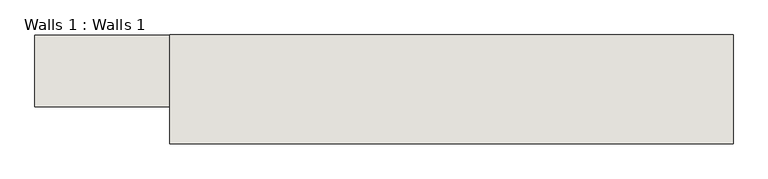
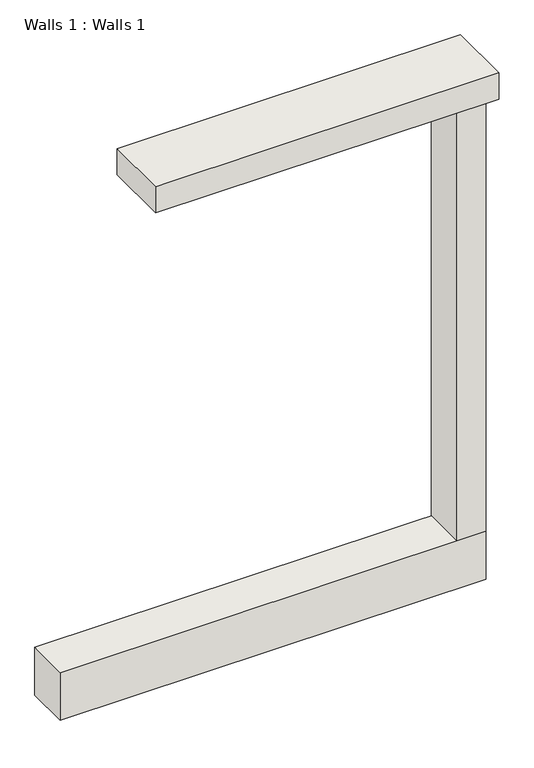
"""IFC4 building model written with IfcOpenShell, lengths in millimetres: wall geometry, Walls 1 : Walls 1."""

from ifc_helpers import new_model, si_unit, frame, origin, place, context, project, spatial, polyline, outline, extrude, source, transform, mapped, element, save


def walls_1_walls_1_d5e167dd(model_context):
    return source(origin(), model_context, "Body", "SweptSolid", [
        extrude(outline(polyline([(-157.3821198, 847.4330681), (-5949.9629707, 847.4330681), (-5949.9629707, 1442.2720741), (-157.3821198, 1442.2720741), (-157.3821198, 847.4330681)])), frame((0.0, 0.0, 3657.6), z_axis=(0.0, 0.0, 1.0), x_axis=(1.0, 0.0, 0.0)), (0.0, 0.0, 1.0), 684.1312703),
        extrude(outline(polyline([(-157.3821198, 847.4330681), (-550.3609948, 847.4330681), (-550.3609948, 1442.2720741), (-157.3821198, 1442.2720741), (-157.3821198, 847.4330681)])), frame((0.0, 0.0, 4341.7312703), z_axis=(0.0, 0.0, 1.0), x_axis=(1.0, 0.0, 0.0)), (0.0, 0.0, 1.0), 6402.4687297),
        extrude(outline(polyline([(-157.3821198, 539.80098), (-4830.9821198, 539.80098), (-4830.9821198, 1442.2720741), (-157.3821198, 1442.2720741), (-157.3821198, 539.80098)])), frame((0.0, 0.0, 10744.2), z_axis=(0.0, 0.0, 1.0), x_axis=(1.0, 0.0, 0.0)), (0.0, 0.0, 1.0), 375.3451788),
    ])


if __name__ == "__main__":
    model = new_model("IFC4")
    model_context = context("Model", 3, world=origin())
    ifc_project = project(units=[si_unit("LENGTHUNIT", "METRE", prefix="MILLI")], contexts=[model_context])
    site = spatial("IfcSite", under=ifc_project)
    building = spatial("IfcBuilding", under=site)
    placement = place(None, origin())
    walls_1_walls_1_shape = walls_1_walls_1_d5e167dd(model_context)
    element("IfcWall", 1, ObjectType="Walls 1 : Walls 1", at=placement, inside=building, context=model_context, shape_type="MappedRepresentation", body=[
        mapped(walls_1_walls_1_shape, transform((0.0, 0.0, 0.0), x_axis=(1.0, 0.0, 0.0), y_axis=(0.0, 1.0, 0.0), z_axis=(0.0, 0.0, 1.0))),
    ])
    save(model, "model.ifc")

# Revit data of these elements
# Element 1 (IfcWall, "Walls 1 : Walls 1")
#   Materials on its faces: "Default Wall"
# Materials
#   "Default Wall": colour RGB 128 128 128, transparency 0
